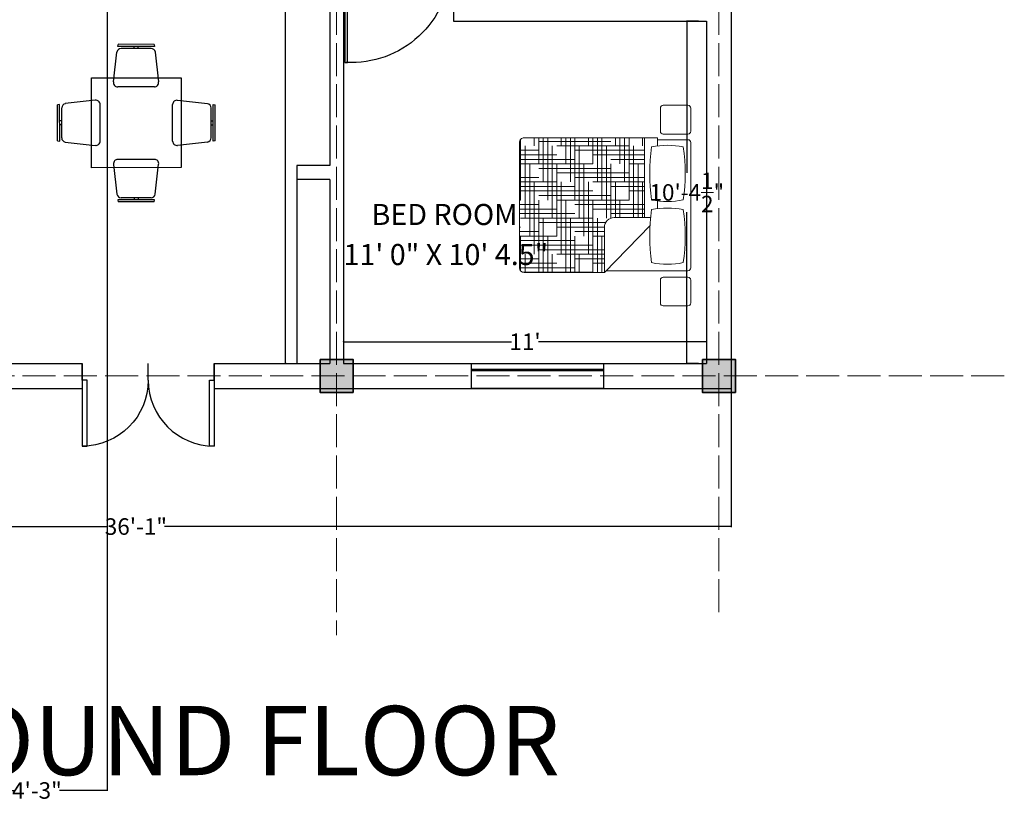
# Model space of a CAD drawing. Units: inches. Extents: x -113 to 5399, y -1393 to 3302.
# Tile 3 of 40: x 1068 to 1427, y -14 to 271. Entities that reach past the tile are written whole.
import ezdxf

# ---------------------------------------------------------------- set-up
doc = ezdxf.new("R2010")
doc.units = ezdxf.units.IN
doc.header["$MEASUREMENT"] = 0
doc.linetypes.add('ACAD_ISO02W100', pattern=[15, 12, -3])
for name, color, linetype, lineweight in [('A-ANNO-DIMS', 254, 'Continuous', 18), ('A-ANNO-TEXT', 7, 'Continuous', 25), ('A-AREA-IDEN', 4, 'Continuous', 18), ('A-COLS', 7, 'Continuous', 35), ('doors', 2, 'Continuous', 25), ('furniture', 131, 'Continuous', 18), ('GRIDS', 7, 'ACAD_ISO02W100', 13), ('walls', 1, 'Continuous', 25), ('windows', 3, 'Continuous', 25)]:
    doc.layers.add(name, color=color, linetype=linetype, lineweight=lineweight)
doc.layers.add('B-FURNITURE', color=22, linetype='Continuous')
doc.styles.get("Standard").update_dxf_attribs({"font": 'arial.ttf'})
doc.dimstyles.get("Standard").update_dxf_attribs({"dimtxt": 6, "dimasz": 0.18, "dimexe": 0.18, "dimexo": 0.0625, "dimgap": 0.09, "dimtad": 0, "dimtih": 1, "dimtoh": 1, "dimdec": 1, "dimzin": 0, "dimdsep": 46, "dimlunit": 4, "dimtxsty": 'Standard', "dimblk": 'ARCHTICK', "dimcen": 0.09, "dimadec": 0, "dimazin": 0, "dimtfac": 1, "dimtdec": 1, "dimtofl": 0, "dimtmove": 0, "dimatfit": 3, "dimfxl": 1, "dimtolj": 1, "dimtzin": 0, "dimarcsym": 0})

# ---------------------------------------------------------------- blocks, each defined once
blk = doc.blocks.new('*U2')
for p, q in [((0, 0), (0, -6)), ((24, 0), (24, -6))]:
    blk.add_line(p, q)
blk.add_lwpolyline([(0, 0), (0, 24), (1.75, 24), (1.75, 0)], close=True)
blk.add_arc((0, 0), 24, 0, 90)
blk = doc.blocks.new('*X4')
at = {"color": 0}
for p, q in [((4.359, 18.562), (4.359, 18.646)), ((4.5, 18), (4.5, 18.646)), ((4.547, 18.188), (4.547, 18.646)), ((4.594, 18.375), (4.594, 18.646)), ((4.641, 18.562), (4.641, 18.646)), ((4.687, 18.609), (5.437, 18.609)), ((4.781, 18), (4.781, 18.646)), ((4.828, 18.188), (4.828, 18.646)), ((4.875, 18.375), (4.875, 18.646)), ((4.922, 18.562), (4.922, 18.646)), ((5.062, 18), (5.062, 18.646)), ((5.109, 18.188), (5.109, 18.646)), ((5.156, 18.375), (5.156, 18.646)), ((5.203, 18.562), (5.203, 18.646)), ((5.344, 18), (5.344, 18.646)), ((5.391, 18.188), (5.391, 18.646)), ((5.437, 18.375), (5.437, 18.646)), ((5.484, 18.562), (5.484, 18.646)), ((5.625, 18), (5.625, 18.629)), ((4.34, 18.516), (5.062, 18.516)), ((4.453, 17.817), (4.453, 18.562)), ((4.5, 18.562), (5.25, 18.562)), ((4.734, 17.812), (4.734, 18.562)), ((5.016, 17.812), (5.016, 18.562)), ((5.297, 17.812), (5.297, 18.562)), ((5.437, 18.516), (5.637, 18.516)), ((5.578, 17.812), (5.578, 18.562)), ((5.625, 18.562), (5.637, 18.562)), ((4.34, 18.469), (4.875, 18.469)), ((4.34, 18.422), (4.687, 18.422)), ((5.062, 18.422), (5.637, 18.422)), ((5.25, 18.469), (5.637, 18.469)), ((4.34, 18.375), (4.5, 18.375)), ((4.406, 17.817), (4.406, 18.375)), ((4.687, 18.328), (5.437, 18.328)), ((4.687, 17.811), (4.687, 18.375)), ((4.875, 18.375), (5.625, 18.375)), ((4.969, 17.625), (4.969, 18.375)), ((5.25, 17.625), (5.25, 18.375)), ((5.531, 17.625), (5.531, 18.375)), ((4.34, 18.234), (5.062, 18.234)), ((4.5, 18.281), (5.25, 18.281)), ((5.437, 18.234), (5.637, 18.234)), ((5.625, 18.281), (5.637, 18.281)), ((4.34, 18.188), (4.875, 18.188)), ((4.34, 18.141), (4.687, 18.141)), ((4.359, 17.817), (4.359, 18.188)), ((4.641, 17.817), (4.641, 18.188)), ((4.922, 17.438), (4.922, 18.188)), ((5.062, 18.141), (5.637, 18.141)), ((5.203, 17.438), (5.203, 18.188)), ((5.25, 18.188), (5.637, 18.188)), ((5.484, 17.438), (5.484, 18.188)), ((4.34, 18.094), (4.5, 18.094)), ((4.5, 18), (5.25, 18)), ((4.594, 17.817), (4.594, 18)), ((4.687, 18.047), (5.437, 18.047)), ((4.875, 18.094), (5.625, 18.094)), ((4.875, 17.25), (4.875, 18)), ((5.156, 17.25), (5.156, 18)), ((5.437, 17.25), (5.437, 18)), ((5.625, 18), (5.637, 18)), ((4.34, 17.953), (5.062, 17.953)), ((4.34, 17.906), (4.875, 17.906)), ((5.25, 17.906), (5.637, 17.906)), ((5.437, 17.953), (5.637, 17.953)), ((4.34, 17.859), (4.687, 17.859)), ((4.828, 17.246), (4.828, 17.812)), ((4.875, 17.812), (5.625, 17.812)), ((5.062, 17.859), (5.637, 17.859)), ((5.109, 17.246), (5.109, 17.812)), ((5.391, 17.246), (5.391, 17.812)), ((4.742, 17.766), (5.437, 17.766)), ((4.755, 17.719), (5.25, 17.719)), ((5.625, 17.719), (5.637, 17.719)), ((4.755, 17.672), (5.062, 17.672)), ((4.755, 17.625), (4.875, 17.625)), ((4.781, 17.246), (4.781, 17.625)), ((5.062, 17.246), (5.062, 17.625)), ((5.25, 17.625), (5.637, 17.625)), ((5.344, 17.246), (5.344, 17.625)), ((5.437, 17.672), (5.637, 17.672)), ((5.625, 17.263), (5.625, 17.625)), ((4.755, 17.484), (5.437, 17.484)), ((4.875, 17.531), (5.625, 17.531)), ((5.062, 17.578), (5.637, 17.578)), ((4.755, 17.438), (5.25, 17.438)), ((4.755, 17.391), (5.062, 17.391)), ((5.016, 17.246), (5.016, 17.438)), ((5.297, 17.246), (5.297, 17.438)), ((5.437, 17.391), (5.637, 17.391)), ((5.578, 17.246), (5.578, 17.438)), ((5.625, 17.438), (5.637, 17.438)), ((4.755, 17.344), (4.875, 17.344)), ((5.062, 17.297), (5.637, 17.297)), ((5.25, 17.344), (5.637, 17.344)), ((4.875, 17.25), (5.608, 17.25)), ((4.969, 17.246), (4.969, 17.25)), ((5.25, 17.246), (5.25, 17.25)), ((5.531, 17.246), (5.531, 17.25))]:
    blk.add_line(p, q, dxfattribs=at)
blk = doc.blocks.new('MAT-P01')
for p, q in [((0.009, 0.846), (0.247, 0.846)), ((0.374, 0.846), (1.674, 0.846)), ((1.792, 0.846), (2.031, 0.846)), ((-0.021, 0.816), (-0.021, 0.56)), ((0.277, 0.816), (0.277, 0.56)), ((0.344, 0.816), (0.344, -0.032)), ((1.704, 0.816), (1.704, 0.5)), ((1.762, 0.816), (1.762, 0.56)), ((2.061, 0.816), (2.061, 0.56)), ((0.009, 0.53), (0.247, 0.53)), ((1.792, 0.53), (2.031, 0.53)), ((0.815, 0.423), (0.324, -0.051)), ((0.895, 0.429), (0.895, 0.049)), ((0.988, 0.5), (1.069, 0.5)), ((1.639, 0.5), (1.724, 0.5)), ((1.724, 0.5), (1.724, -0.884)), ((0.895, 0.364), (1.724, 0.364)), ((0.895, 0.364), (0.895, 0.049)), ((0.895, 0.364), (1.724, 0.364)), ((1.724, 0.364), (1.724, -0.884)), ((0.324, -0.051), (0.795, -0.051)), ((0.324, -0.051), (0.324, -0.884)), ((0.374, -0.934), (1.674, -0.934))]:
    blk.add_line(p, q)
for centre, radius, start, end in [((0.009, 0.816), 0.03, 90, 180), ((0.247, 0.816), 0.03, 0, 90), ((0.374, 0.816), 0.03, 90, 180), ((1.674, 0.816), 0.03, 0, 90), ((1.792, 0.816), 0.03, 90, 180), ((2.031, 0.816), 0.03, 0, 90), ((1.225, 0.603), 0.814, 168.373, 191.627), ((0.703, -1.144), 1.931, 81.8162, 98.1838), ((0.181, 0.603), 0.814, 348.373, 11.627), ((1.877, 0.603), 0.814, 168.373, 191.627), ((1.354, -1.144), 1.931, 81.8162, 98.1838), ((0.832, 0.603), 0.814, 348.373, 11.627), ((0.009, 0.56), 0.03, 180, 270), ((0.247, 0.56), 0.03, 270, 0), ((1.792, 0.56), 0.03, 180, 270), ((2.031, 0.56), 0.03, 270, 0), ((0.703, 2.35), 1.931, 261.8162, 278.1838), ((1.354, 2.35), 1.931, 261.8162, 278.1838), ((0.795, 0.049), 0.1, 270, 0), ((0.374, -0.884), 0.05, 180, 270), ((1.674, -0.884), 0.05, 270, 0)]:
    blk.add_arc(centre, radius, start, end)
at = {"rotation": 270}
blk.add_blockref('*X4', (-16.922, 4.704), dxfattribs=at)
blk = doc.blocks.new('A$C6ACA79D1')
at = {"layer": 'B-FURNITURE'}
for p, q in [((-0.503, 0.053), (-0.801, -0.244)), ((-0.483, 0.039), (-0.787, -0.264)), ((-0.503, 0.053), (-0.483, 0.039)), ((-0.429, 0), (-0.155, -0.22)), ((0.787, -0.259), (0.483, 0.044)), ((0.484, 0.043), (0.504, 0.058)), ((0.743, -0.249), (0.493, 0)), ((0.801, -0.239), (0.503, 0.059)), ((-0.493, -0.005), (-0.743, -0.254)), ((-0.601, -0.112), (-0.618, -0.095)), ((0.601, -0.107), (0.618, -0.09)), ((-0.635, -0.147), (-0.652, -0.13)), ((0.635, -0.142), (0.652, -0.124)), ((-0.786, -0.264), (-0.8, -0.244)), ((-0.148, -0.296), (-0.451, -0.599)), ((0.451, -0.594), (0.148, -0.291)), ((0.748, -0.313), (0.527, -0.588)), ((0.801, -0.239), (0.787, -0.259)), ((-0.148, -1.194), (-0.451, -0.891)), ((0.451, -0.896), (0.148, -1.199)), ((0.748, -1.177), (0.527, -0.902)), ((-0.503, -1.544), (-0.801, -1.246)), ((-0.786, -1.227), (-0.8, -1.247)), ((-0.483, -1.529), (-0.787, -1.226)), ((-0.493, -1.485), (-0.743, -1.236)), ((0.787, -1.231), (0.483, -1.535)), ((0.743, -1.241), (0.493, -1.49)), ((0.801, -1.251), (0.503, -1.549)), ((0.801, -1.251), (0.787, -1.231)), ((-0.635, -1.343), (-0.652, -1.361)), ((-0.601, -1.378), (-0.618, -1.395)), ((-0.429, -1.49), (-0.155, -1.27)), ((0.601, -1.383), (0.618, -1.4)), ((0.635, -1.349), (0.652, -1.366)), ((-0.503, -1.544), (-0.483, -1.529)), ((0.484, -1.534), (0.504, -1.548))]:
    blk.add_line(p, q, dxfattribs=at)
at = {"layer": 'B-FURNITURE', "ltscale": 300}
for p, q in [((0.155, -0.215), (0.429, 0.005)), ((-0.527, -0.593), (-0.748, -0.319)), ((-0.527, -0.897), (-0.748, -1.172)), ((0.155, -1.275), (0.429, -1.496))]:
    blk.add_line(p, q, dxfattribs=at)
blk.add_lwpolyline([(-0.742, -0.742), (0, 0), (0.742, -0.742), (0, -1.485)], close=True, dxfattribs=at)
at = {"layer": 'B-FURNITURE', "ltscale": 400}
for centre, start, end in [((-0.458, -0.04), 54.4069, 135), ((0.459, -0.036), 45, 125.5931), ((-0.706, -0.289), 135, 215.5931), ((0.707, -0.284), 324.4069, 45), ((-0.706, -1.201), 144.4069, 225), ((0.707, -1.206), 315, 35.5931), ((-0.458, -1.45), 225, 305.5931), ((0.459, -1.454), 234.4069, 315)]:
    blk.add_arc(centre, 0.0499, start, end, dxfattribs=at)
at = {"layer": 'B-FURNITURE', "ltscale": 300}
for centre, start, end in [((-0.184, -0.261), 315, 54.4069), ((0.184, -0.256), 125.5931, 225), ((-0.487, -0.564), 215.5931, 315), ((0.487, -0.559), 225, 324.4069), ((-0.487, -0.926), 45, 144.4069), ((0.487, -0.931), 35.5931, 135), ((-0.184, -1.229), 305.5931, 45), ((0.184, -1.234), 135, 234.4069)]:
    blk.add_arc(centre, 0.05, start, end, dxfattribs=at)
blk = doc.blocks.new('_ArchTick')
at = {"color": 0, "linetype": 'ByBlock', "const_width": 0.15}
blk.add_lwpolyline([(-0.5, -0.5), (0.5, 0.5)], dxfattribs=at)
blk = doc.blocks.new('*D21')
at = {"layer": 'A-ANNO-DIMS', "color": 0, "lineweight": -2, "transparency": 16777216}
for p, q in [((894.23, 136.47), (894.23, 86.09)), ((1327.23, 136.47), (1327.23, 86.09)), ((894.23, 86.27), (1100.34, 86.27)), ((1327.23, 86.27), (1121.12, 86.27))]:
    blk.add_line(p, q, dxfattribs=at)
at = {"layer": 'Defpoints', "color": 0, "transparency": 16777216}
for p in [(894.23, 136.53), (1327.23, 136.53), (1327.23, 86.27)]:
    blk.add_point(p, dxfattribs=at)
at = {"layer": 'A-ANNO-DIMS', "color": 0, "lineweight": -2, "transparency": 16777216, "xscale": 0.18, "yscale": 0.18, "zscale": 0.18, "rotation": 180}
blk.add_blockref('_ArchTick', (894.23, 86.27), dxfattribs=at)
at = {"layer": 'A-ANNO-DIMS', "color": 0, "lineweight": -2, "transparency": 16777216, "xscale": 0.18, "yscale": 0.18, "zscale": 0.18}
blk.add_blockref('_ArchTick', (1327.23, 86.27), dxfattribs=at)
at = {"layer": 'A-ANNO-DIMS', "color": 0, "transparency": 16777216, "insert": (1110.73, 86.27), "char_height": 6, "attachment_point": 5}
blk.add_mtext('\\A1;36\'-1"', dxfattribs=at)
blk = doc.blocks.new('*D27')
at = {"layer": 'A-ANNO-DIMS', "color": 0, "lineweight": -2, "transparency": 16777216}
for p, q in [((1165.42, 416.53), (1164.91, 416.53)), ((1165.09, 416.53), (1165.09, 284.13)), ((1165.09, 145.53), (1165.09, 277.93)), ((1165.42, 145.53), (1164.91, 145.53))]:
    blk.add_line(p, q, dxfattribs=at)
at = {"layer": 'Defpoints', "color": 0, "transparency": 16777216}
for p in [(1165.48, 416.53), (1165.09, 145.53), (1165.48, 145.53)]:
    blk.add_point(p, dxfattribs=at)
at = {"layer": 'A-ANNO-DIMS', "color": 0, "lineweight": -2, "transparency": 16777216, "xscale": 0.18, "yscale": 0.18, "zscale": 0.18}
for p, rotation in [((1165.09, 416.53), 90), ((1165.09, 145.53), 270)]:
    blk.add_blockref('_ArchTick', p, dxfattribs=dict(at, rotation=rotation))
at = {"layer": 'A-ANNO-DIMS', "color": 0, "transparency": 16777216, "insert": (1165.09, 281.03), "char_height": 6, "attachment_point": 5}
blk.add_mtext('\\A1;22\'-7"', dxfattribs=at)
blk = doc.blocks.new('*D37')
at = {"layer": 'A-ANNO-DIMS', "color": 0, "lineweight": -2, "transparency": 16777216}
for p, q in [((1186.23, 153.54), (1186.23, 153.66)), ((1186.23, 153.48), (1247.33, 153.48)), ((1318.23, 153.48), (1257.13, 153.48)), ((1318.23, 153.54), (1318.23, 153.66))]:
    blk.add_line(p, q, dxfattribs=at)
at = {"layer": 'Defpoints', "color": 0, "transparency": 16777216}
for p in [(1186.23, 153.48), (1186.23, 153.48), (1318.23, 153.48)]:
    blk.add_point(p, dxfattribs=at)
at = {"layer": 'A-ANNO-DIMS', "color": 0, "lineweight": -2, "transparency": 16777216, "xscale": 0.18, "yscale": 0.18, "zscale": 0.18, "rotation": 180}
blk.add_blockref('_ArchTick', (1186.23, 153.48), dxfattribs=at)
at = {"layer": 'A-ANNO-DIMS', "color": 0, "lineweight": -2, "transparency": 16777216, "xscale": 0.18, "yscale": 0.18, "zscale": 0.18}
blk.add_blockref('_ArchTick', (1318.23, 153.48), dxfattribs=at)
at = {"layer": 'A-ANNO-DIMS', "color": 0, "transparency": 16777216, "insert": (1252.23, 153.48), "char_height": 6, "attachment_point": 5}
blk.add_mtext("\\A1;11'", dxfattribs=at)
blk = doc.blocks.new('*D38')
at = {"layer": 'A-ANNO-DIMS', "color": 0, "lineweight": -2, "transparency": 16777216}
for p, q in [((1315.34, 270.03), (1310.91, 270.03)), ((1311.09, 270.03), (1311.09, 214.95)), ((1311.09, 145.53), (1311.09, 200.62)), ((1315.34, 145.53), (1310.91, 145.53))]:
    blk.add_line(p, q, dxfattribs=at)
at = {"layer": 'Defpoints', "color": 0, "transparency": 16777216}
for p in [(1315.4, 270.03), (1311.09, 145.53), (1315.4, 145.53)]:
    blk.add_point(p, dxfattribs=at)
at = {"layer": 'A-ANNO-DIMS', "color": 0, "lineweight": -2, "transparency": 16777216, "xscale": 0.18, "yscale": 0.18, "zscale": 0.18}
for p, rotation in [((1311.09, 270.03), 90), ((1311.09, 145.53), 270)]:
    blk.add_blockref('_ArchTick', p, dxfattribs=dict(at, rotation=rotation))
at = {"layer": 'A-ANNO-DIMS', "color": 0, "transparency": 16777216, "insert": (1311.09, 207.78), "char_height": 6, "attachment_point": 5}
blk.add_mtext('\\A1;10\'-4{\\H1x;\\S1/2;}"', dxfattribs=at)
blk = doc.blocks.new('WIN-PLAN-48IN')
h = blk.add_hatch(color=256)
h.dxf.hatch_style = 1
h.paths.add_polyline_path([(48, 2.5), (0, 2.5), (0, 2), (48, 2)])
for p, q in [((0, 9), (48, 9)), ((0, 0), (0, 9)), ((48, 9), (48, 0)), ((48, 2.5), (0, 2.5)), ((48, 2), (0, 2)), ((48, 0), (0, 0))]:
    blk.add_line(p, q)
blk = doc.blocks.new('COLUMN-12IN-SQUARE')
h = blk.add_hatch(color=256)
h.dxf.hatch_style = 1
h.paths.add_polyline_path([(6, 6), (-6, 6), (-6, -6), (6, -6)])
blk.add_lwpolyline([(-6, 6), (6, 6), (6, -6), (-6, -6)], close=True)
blk = doc.blocks.new('DOOR-SINGLE-36IN-PLAN')
for p, q in [((0.5, 2), (0.5, 36.98)), ((0.5, 36.98), (1.5, 36.98)), ((1.5, 36.98), (1.5, 2)), ((0, 2), (0, 0)), ((0, 2), (1.04, 2)), ((1.5, 2), (0.5, 2)), ((1.04, 2), (1.04, 0.98)), ((1.04, 0.98), (2, 0.98)), ((2, 0), (2, 0.98)), ((38.96, 0.98), (38, 0.98)), ((38, 0), (38, 0.98)), ((40, 2), (38.96, 2)), ((38.96, 2), (38.96, 0.98)), ((40, 0), (40, 2)), ((0, 0), (2, 0)), ((0, 0), (2, 0)), ((38, 0), (40, 0))]:
    blk.add_line(p, q)
blk.add_arc((2.94, 0.99), 36.04, 1.6003, 93.0893)
blk = doc.blocks.new('*D212')
at = {"layer": 'A-ANNO-DIMS', "color": 0, "lineweight": -2, "transparency": 16777216}
for p, q in [((1049.23, 425.47), (1049.23, -9.87)), ((1100.23, 425.47), (1100.23, -9.87)), ((1049.23, -9.69), (1066.55, -9.69)), ((1100.23, -9.69), (1082.92, -9.69))]:
    blk.add_line(p, q, dxfattribs=at)
at = {"layer": 'Defpoints', "color": 0, "transparency": 16777216}
for p in [(1049.23, 425.53), (1100.23, 425.53), (1100.23, -9.69)]:
    blk.add_point(p, dxfattribs=at)
at = {"layer": 'A-ANNO-DIMS', "color": 0, "lineweight": -2, "transparency": 16777216, "xscale": 0.18, "yscale": 0.18, "zscale": 0.18, "rotation": 180}
blk.add_blockref('_ArchTick', (1049.23, -9.69), dxfattribs=at)
at = {"layer": 'A-ANNO-DIMS', "color": 0, "lineweight": -2, "transparency": 16777216, "xscale": 0.18, "yscale": 0.18, "zscale": 0.18}
blk.add_blockref('_ArchTick', (1100.23, -9.69), dxfattribs=at)
at = {"layer": 'A-ANNO-DIMS', "color": 0, "transparency": 16777216, "insert": (1074.73, -9.69), "char_height": 6, "attachment_point": 5}
blk.add_mtext('\\A1;4\'-3"', dxfattribs=at)

msp = doc.modelspace()

# ---------------------------------------------------------------- linework, layer by layer
at = {"layer": 'GRIDS'}
for p, q in [((1183.73, 922.09), (1183.73, 46.81)), ((1322.73, 922.09), (1322.73, 54.5)), ((1426.54, 141.03), (768.3, 141.03))]:
    msp.add_line(p, q, dxfattribs=at)
at = {"layer": 'walls'}
for p, q in [((1327.23, 786.53), (1327.23, 136.53)), ((1226.23, 299.03), (1226.23, 270.03)), ((1181.23, 292.03), (1181.23, 217.53)), ((1186.23, 292.03), (1186.23, 145.53)), ((1226.23, 270.03), (1318.23, 270.03)), ((1318.23, 270.03), (1318.23, 145.53)), ((1181.23, 217.53), (1169.23, 217.53)), ((1169.23, 217.53), (1169.23, 212.53)), ((1181.23, 212.53), (1169.23, 212.53)), ((1169.23, 212.53), (1169.23, 145.53)), ((1181.23, 212.53), (1181.23, 145.53)), ((1049.23, 145.53), (1091.23, 145.53)), ((1091.23, 145.53), (1091.23, 136.53)), ((1139.23, 145.53), (1139.23, 136.53)), ((1139.23, 145.53), (1181.23, 145.53)), ((1186.23, 145.53), (1318.23, 145.53)), ((894.23, 136.53), (1091.23, 136.53)), ((1139.23, 136.53), (1232.73, 136.53)), ((1186.23, 136.53), (1327.23, 136.53))]:
    msp.add_line(p, q, dxfattribs=at)

# ---------------------------------------------------------------- block references
at = {"layer": 'A-COLS'}
for p in [(1183.73, 141.03), (1322.73, 141.03)]:
    msp.add_blockref('COLUMN-12IN-SQUARE', p, dxfattribs=at)
at = {"layer": 'doors', "extrusion": (0, 0, -1), "zscale": -1, "rotation": 180}
msp.add_blockref('DOOR-SINGLE-36IN-PLAN', (-1186.23, 292.03), dxfattribs=at)
at = {"layer": 'doors', "xscale": -1, "rotation": 180}
msp.add_blockref('*U2', (1091.23, 139.53), dxfattribs=at)
at = {"layer": 'doors', "rotation": 180}
msp.add_blockref('*U2', (1139.23, 139.53), dxfattribs=at)
at = {"layer": 'furniture'}
for name, p, xscale, yscale, zscale, rotation in [('A$C6ACA79D1', (1127.22, 249.39), 31.0665876167328, 31.0665876167328, 31.0665876167328, 314.9999999999397), ('MAT-P01', (1282.91, 167.26), -35.02364872074636, 35.02364872074636, 35.02364872074636, 270)]:
    msp.add_blockref(name, p, dxfattribs=dict(at, xscale=xscale, yscale=yscale, zscale=zscale, rotation=rotation))
at = {"layer": 'windows', "rotation": 180}
msp.add_blockref('WIN-PLAN-48IN', (1280.73, 145.53), dxfattribs=at)

# ---------------------------------------------------------------- texts
at = {"layer": 'A-ANNO-TEXT'}
msp.add_text('GROUND FLOOR', height=25.17, dxfattribs=at).set_placement((1002.73, -4.13))
at = {"layer": 'A-AREA-IDEN'}
for s, height, p in [('BED ROOM', 7.647, (1196.42, 195.93)), ('11\' 0" X 10\' 4.5"', 7.6473, (1186.23, 181.37))]:
    msp.add_text(s, height=height, dxfattribs=at).set_placement(p)

# ---------------------------------------------------------------- dimensions: what is measured, and where the dimension line sits
at = {"layer": 'A-ANNO-DIMS'}
for base, p1, p2, override, picture, middle in [((1100.23, -9.69), (1049.23, 425.53), (1100.23, 425.53), {"dimdec": 1, "dimlfac": 1, "dimrnd": 0, "dimzin": 1, "dimdsep": 46, "dimlunit": 4, "dimfrac": 2}, '*D212', (1074.73, -9.69)), ((1186.23, 153.48), (1318.23, 153.48), (1186.23, 153.48), {"dimclrd": 0, "dimclre": 0, "dimclrt": 0}, '*D37', (1252.23, 153.48)), ((1327.23, 86.27), (894.23, 136.53), (1327.23, 136.53), {"dimclrd": 0, "dimclre": 0, "dimclrt": 0}, '*D21', (1110.73, 86.27))]:
    dim = msp.add_linear_dim(base=base, p1=p1, p2=p2, dimstyle='Standard', override=override, dxfattribs=at)
    dim.commit()
    dim.dimension.update_dxf_attribs({"geometry": picture, "text_midpoint": middle})
for base, p1, p2, picture, middle in [((1165.09, 145.53), (1165.48, 416.53), (1165.48, 145.53), '*D27', (1165.09, 281.03)), ((1311.09, 145.53), (1315.4, 270.03), (1315.4, 145.53), '*D38', (1311.09, 207.78))]:
    dim = msp.add_linear_dim(base=base, p1=p1, p2=p2, angle=90, dimstyle='Standard', override={"dimclrd": 0, "dimclre": 0, "dimclrt": 0}, dxfattribs=at)
    dim.commit()
    dim.dimension.update_dxf_attribs({"geometry": picture, "text_midpoint": middle})

doc.saveas('drawing.dxf')
